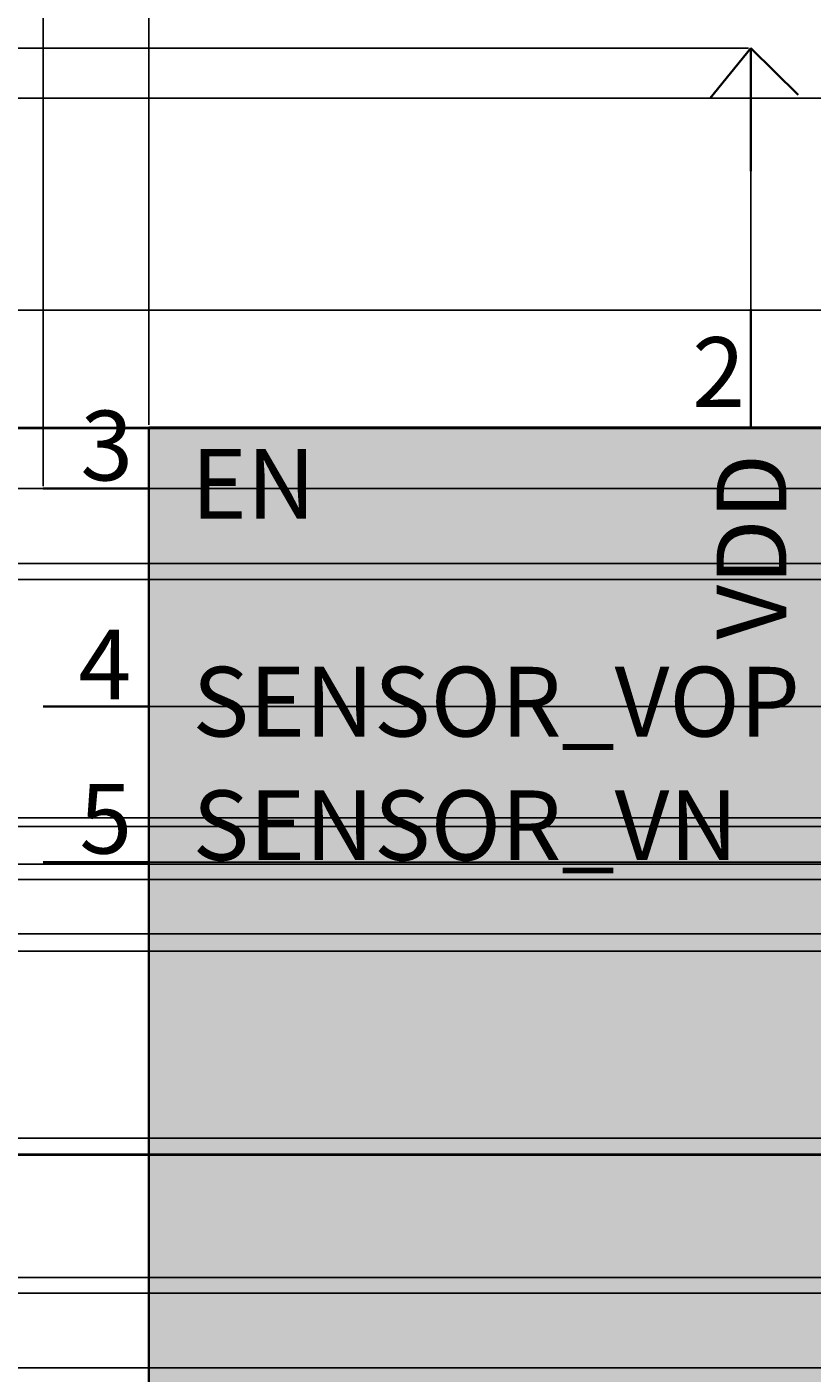
# Model space of a CAD drawing. Units: inches. Extents: x 23 to 132, y 5 to 105.
# Tile 4 of 14: x 47 to 66, y 54 to 87. Entities that reach past the tile are written whole.
import ezdxf

# ---------------------------------------------------------------- set-up
doc = ezdxf.new("R2010")
doc.units = ezdxf.units.IN
doc.header["$MEASUREMENT"] = 0
for name, color, linetype, lineweight in [('A-ANNO-DIMS', 2, 'Continuous', 18), ('E-ANNO-TEXT', 3, 'Continuous', 18), ('E-SYMB', 1, 'Continuous', 35), ('E-SYMB-PATT', 1, 'Continuous', 18), ('E-WIRE', 3, 'Continuous', 25)]:
    doc.layers.add(name, color=color, linetype=linetype, lineweight=lineweight)
doc.styles.get("Standard").update_dxf_attribs({"font": 'arial.ttf'})
doc.dimstyles.get("Standard").update_dxf_attribs({"dimtxt": 0.18, "dimasz": 0.18, "dimexe": 0.18, "dimexo": 0.0625, "dimgap": 0.09, "dimtad": 0, "dimtih": 1, "dimtoh": 1, "dimdec": 4, "dimzin": 0, "dimdsep": 46, "dimtxsty": 'Standard', "dimcen": 0.09, "dimadec": 0, "dimazin": 0, "dimtfac": 1, "dimtdec": 4, "dimtofl": 0, "dimtmove": 0, "dimatfit": 3, "dimfxl": 1, "dimtolj": 1, "dimtzin": 0, "dimarcsym": 0})

# ---------------------------------------------------------------- blocks, each defined once
blk = doc.blocks.new('*D2')
at = {"layer": 'A-ANNO-DIMS', "color": 0, "lineweight": -2, "transparency": 16777216}
for p, q in [((28.697, 66.272), (28.697, 105.232)), ((28.877, 105.052), (75.577, 105.052)), ((123.031, 105.052), (76.33, 105.052)), ((123.211, 99.539), (123.211, 105.232))]:
    blk.add_line(p, q, dxfattribs=at)
at = {"layer": 'A-ANNO-DIMS', "color": 0, "transparency": 16777216}
for points in [[(28.877, 105.082), (28.877, 105.022), (28.697, 105.052)], [(123.031, 105.082), (123.031, 105.022), (123.211, 105.052)]]:
    blk.add_solid(points, dxfattribs=at)
at = {"layer": 'Defpoints', "color": 0, "transparency": 16777216}
for p in [(123.211, 105.052), (123.211, 99.477), (28.697, 66.21)]:
    blk.add_point(p, dxfattribs=at)
at = {"layer": 'A-ANNO-DIMS', "color": 0, "transparency": 16777216, "insert": (75.954, 105.052), "char_height": 0.18, "attachment_point": 5}
blk.add_mtext('\\A1;94.51', dxfattribs=at)
blk = doc.blocks.new('*D6')
at = {"layer": 'A-ANNO-DIMS', "color": 0, "lineweight": -2, "transparency": 16777216}
for p, q in [((50.202, 77.095), (22.942, 77.095)), ((23.122, 76.915), (23.122, 47.733)), ((23.122, 18.187), (23.122, 47.369)), ((50.202, 18.007), (22.942, 18.007))]:
    blk.add_line(p, q, dxfattribs=at)
at = {"layer": 'A-ANNO-DIMS', "color": 0, "transparency": 16777216}
for points in [[(23.092, 76.915), (23.152, 76.915), (23.122, 77.095)], [(23.092, 18.187), (23.152, 18.187), (23.122, 18.007)]]:
    blk.add_solid(points, dxfattribs=at)
at = {"layer": 'Defpoints', "color": 0, "transparency": 16777216}
for p in [(23.122, 77.095), (50.265, 77.095), (50.265, 18.007)]:
    blk.add_point(p, dxfattribs=at)
at = {"layer": 'A-ANNO-DIMS', "color": 0, "transparency": 16777216, "insert": (23.122, 47.551), "char_height": 0.18, "attachment_point": 5}
blk.add_mtext('\\A1;59.09', dxfattribs=at)
blk = doc.blocks.new('*D7')
at = {"layer": 'A-ANNO-DIMS', "color": 0, "lineweight": -2, "transparency": 16777216}
for p, q in [((30.295, 73.877), (30.295, 105.232)), ((30.475, 105.052), (39.895, 105.052)), ((50.085, 105.052), (40.665, 105.052)), ((50.265, 77.157), (50.265, 105.232))]:
    blk.add_line(p, q, dxfattribs=at)
at = {"layer": 'A-ANNO-DIMS', "color": 0, "transparency": 16777216}
for points in [[(30.475, 105.082), (30.475, 105.022), (30.295, 105.052)], [(50.085, 105.082), (50.085, 105.022), (50.265, 105.052)]]:
    blk.add_solid(points, dxfattribs=at)
at = {"layer": 'Defpoints', "color": 0, "transparency": 16777216}
for p in [(50.265, 105.052), (50.265, 77.095), (30.295, 73.814)]:
    blk.add_point(p, dxfattribs=at)
at = {"layer": 'A-ANNO-DIMS', "color": 0, "transparency": 16777216, "insert": (40.28, 105.052), "char_height": 0.18, "attachment_point": 5}
blk.add_mtext('\\A1;19.97', dxfattribs=at)
blk = doc.blocks.new('*D12')
at = {"layer": 'A-ANNO-DIMS', "color": 0, "lineweight": -2, "transparency": 16777216}
for p, q in [((64.714, 86.23), (22.942, 86.23)), ((23.122, 86.05), (23.122, 81.845)), ((23.122, 77.275), (23.122, 81.481)), ((64.714, 77.095), (22.942, 77.095))]:
    blk.add_line(p, q, dxfattribs=at)
at = {"layer": 'A-ANNO-DIMS', "color": 0, "transparency": 16777216}
for points in [[(23.092, 86.05), (23.152, 86.05), (23.122, 86.23)], [(23.092, 77.275), (23.152, 77.275), (23.122, 77.095)]]:
    blk.add_solid(points, dxfattribs=at)
at = {"layer": 'Defpoints', "color": 0, "transparency": 16777216}
for p in [(23.122, 86.23), (64.777, 86.23), (64.777, 77.095)]:
    blk.add_point(p, dxfattribs=at)
at = {"layer": 'A-ANNO-DIMS', "color": 0, "transparency": 16777216, "insert": (23.122, 81.663), "char_height": 0.18, "attachment_point": 5}
blk.add_mtext('\\A1;9.135', dxfattribs=at)
blk = doc.blocks.new('*D15')
at = {"layer": 'A-ANNO-DIMS', "color": 0, "lineweight": -2, "transparency": 16777216}
for p, q in [((50.327, 77.095), (129.239, 77.095)), ((129.059, 76.915), (129.059, 76.538)), ((129.059, 75.801), (129.059, 76.177)), ((47.783, 75.621), (129.239, 75.621))]:
    blk.add_line(p, q, dxfattribs=at)
at = {"layer": 'A-ANNO-DIMS', "color": 0, "transparency": 16777216}
for points in [[(129.029, 76.915), (129.089, 76.915), (129.059, 77.095)], [(129.029, 75.801), (129.089, 75.801), (129.059, 75.621)]]:
    blk.add_solid(points, dxfattribs=at)
at = {"layer": 'Defpoints', "color": 0, "transparency": 16777216}
for p in [(50.265, 77.095), (47.72, 75.621), (129.059, 75.621)]:
    blk.add_point(p, dxfattribs=at)
at = {"layer": 'A-ANNO-DIMS', "color": 0, "transparency": 16777216, "insert": (129.059, 76.358), "char_height": 0.18, "attachment_point": 5}
blk.add_mtext('\\A1;1.47', dxfattribs=at)
blk = doc.blocks.new('*D16')
at = {"layer": 'A-ANNO-DIMS', "color": 0, "lineweight": -2, "transparency": 16777216}
for p, q in [((47.783, 75.621), (129.239, 75.621)), ((129.059, 75.441), (129.059, 73.177)), ((129.059, 70.55), (129.059, 72.814)), ((47.783, 70.37), (129.239, 70.37))]:
    blk.add_line(p, q, dxfattribs=at)
at = {"layer": 'A-ANNO-DIMS', "color": 0, "transparency": 16777216}
for points in [[(129.029, 75.441), (129.089, 75.441), (129.059, 75.621)], [(129.029, 70.55), (129.089, 70.55), (129.059, 70.37)]]:
    blk.add_solid(points, dxfattribs=at)
at = {"layer": 'Defpoints', "color": 0, "transparency": 16777216}
for p in [(47.72, 75.621), (47.72, 70.37), (129.059, 70.37)]:
    blk.add_point(p, dxfattribs=at)
at = {"layer": 'A-ANNO-DIMS', "color": 0, "transparency": 16777216, "insert": (129.059, 72.996), "char_height": 0.18, "attachment_point": 5}
blk.add_mtext('\\A1;5.25', dxfattribs=at)
blk = doc.blocks.new('*D17')
at = {"layer": 'A-ANNO-DIMS', "color": 0, "lineweight": -2, "transparency": 16777216}
for p, q in [((47.783, 70.37), (129.239, 70.37)), ((129.059, 70.19), (129.059, 68.678)), ((129.059, 66.801), (129.059, 68.314)), ((47.783, 66.621), (129.239, 66.621))]:
    blk.add_line(p, q, dxfattribs=at)
at = {"layer": 'A-ANNO-DIMS', "color": 0, "transparency": 16777216}
for points in [[(129.029, 70.19), (129.089, 70.19), (129.059, 70.37)], [(129.029, 66.801), (129.089, 66.801), (129.059, 66.621)]]:
    blk.add_solid(points, dxfattribs=at)
at = {"layer": 'Defpoints', "color": 0, "transparency": 16777216}
for p in [(47.72, 70.37), (47.72, 66.621), (129.059, 66.621)]:
    blk.add_point(p, dxfattribs=at)
at = {"layer": 'A-ANNO-DIMS', "color": 0, "transparency": 16777216, "insert": (129.059, 68.496), "char_height": 0.18, "attachment_point": 5}
blk.add_mtext('\\A1;3.75', dxfattribs=at)
blk = doc.blocks.new('*D48')
at = {"layer": 'A-ANNO-DIMS', "color": 0, "lineweight": -2, "transparency": 16777216}
for p, q in [((41.783, 75.637), (41.783, 105.232)), ((41.963, 105.052), (44.358, 105.052)), ((47.54, 105.052), (45.145, 105.052)), ((47.72, 75.683), (47.72, 105.232))]:
    blk.add_line(p, q, dxfattribs=at)
at = {"layer": 'A-ANNO-DIMS', "color": 0, "transparency": 16777216}
for points in [[(41.963, 105.082), (41.963, 105.022), (41.783, 105.052)], [(47.54, 105.082), (47.54, 105.022), (47.72, 105.052)]]:
    blk.add_solid(points, dxfattribs=at)
at = {"layer": 'Defpoints', "color": 0, "transparency": 16777216}
for p in [(47.72, 105.052), (41.783, 75.575), (47.72, 75.621)]:
    blk.add_point(p, dxfattribs=at)
at = {"layer": 'A-ANNO-DIMS', "color": 0, "transparency": 16777216, "insert": (44.752, 105.052), "char_height": 0.18, "attachment_point": 5}
blk.add_mtext('\\A1;5.937', dxfattribs=at)
blk = doc.blocks.new('*D57')
at = {"layer": 'A-ANNO-DIMS', "color": 0, "lineweight": -2, "transparency": 16777216}
for p, q in [((30.358, 64.901), (129.239, 64.901)), ((129.059, 64.721), (129.059, 62.62)), ((129.059, 60.155), (129.059, 62.256)), ((30.358, 59.975), (129.239, 59.975))]:
    blk.add_line(p, q, dxfattribs=at)
at = {"layer": 'A-ANNO-DIMS', "color": 0, "transparency": 16777216}
for points in [[(129.029, 64.721), (129.089, 64.721), (129.059, 64.901)], [(129.029, 60.155), (129.089, 60.155), (129.059, 59.975)]]:
    blk.add_solid(points, dxfattribs=at)
at = {"layer": 'Defpoints', "color": 0, "transparency": 16777216}
for p in [(30.295, 64.901), (129.059, 64.901), (30.295, 59.975)]:
    blk.add_point(p, dxfattribs=at)
at = {"layer": 'A-ANNO-DIMS', "color": 0, "transparency": 16777216, "insert": (129.059, 62.438), "char_height": 0.18, "attachment_point": 5}
blk.add_mtext('\\A1;4.925', dxfattribs=at)
blk = doc.blocks.new('*D58')
at = {"layer": 'A-ANNO-DIMS', "color": 0, "lineweight": -2, "transparency": 16777216}
for p, q in [((30.358, 73.814), (129.239, 73.814)), ((129.059, 73.634), (129.059, 70.194)), ((129.059, 66.39), (129.059, 69.83)), ((30.359, 66.21), (129.239, 66.21))]:
    blk.add_line(p, q, dxfattribs=at)
at = {"layer": 'A-ANNO-DIMS', "color": 0, "transparency": 16777216}
for points in [[(129.029, 73.634), (129.089, 73.634), (129.059, 73.814)], [(129.029, 66.39), (129.089, 66.39), (129.059, 66.21)]]:
    blk.add_solid(points, dxfattribs=at)
at = {"layer": 'Defpoints', "color": 0, "transparency": 16777216}
for p in [(30.295, 73.814), (129.059, 73.814), (30.297, 66.21)]:
    blk.add_point(p, dxfattribs=at)
at = {"layer": 'A-ANNO-DIMS', "color": 0, "transparency": 16777216, "insert": (129.059, 70.012), "char_height": 0.18, "attachment_point": 5}
blk.add_mtext('\\A1;7.604', dxfattribs=at)
blk = doc.blocks.new('*D65')
at = {"layer": 'A-ANNO-DIMS', "color": 0, "lineweight": -2, "transparency": 16777216}
for p, q in [((38.414, 67.485), (129.239, 67.485)), ((129.059, 67.305), (129.059, 66.165)), ((129.059, 64.66), (129.059, 65.801)), ((38.414, 64.48), (129.239, 64.48))]:
    blk.add_line(p, q, dxfattribs=at)
at = {"layer": 'A-ANNO-DIMS', "color": 0, "transparency": 16777216}
for points in [[(129.029, 67.305), (129.089, 67.305), (129.059, 67.485)], [(129.029, 64.66), (129.089, 64.66), (129.059, 64.48)]]:
    blk.add_solid(points, dxfattribs=at)
at = {"layer": 'Defpoints', "color": 0, "transparency": 16777216}
for p in [(38.351, 67.485), (129.059, 67.485), (38.351, 64.48)]:
    blk.add_point(p, dxfattribs=at)
at = {"layer": 'A-ANNO-DIMS', "color": 0, "transparency": 16777216, "insert": (129.059, 65.983), "char_height": 0.18, "attachment_point": 5}
blk.add_mtext('\\A1;3.005', dxfattribs=at)
blk = doc.blocks.new('*D70')
at = {"layer": 'A-ANNO-DIMS', "color": 0, "lineweight": -2, "transparency": 16777216}
for p, q in [((35.392, 56.625), (129.239, 56.625)), ((129.059, 56.445), (129.059, 55.716)), ((129.059, 54.624), (129.059, 55.352)), ((33.892, 54.444), (129.239, 54.444))]:
    blk.add_line(p, q, dxfattribs=at)
at = {"layer": 'A-ANNO-DIMS', "color": 0, "transparency": 16777216}
for points in [[(129.029, 56.445), (129.089, 56.445), (129.059, 56.625)], [(129.029, 54.624), (129.089, 54.624), (129.059, 54.444)]]:
    blk.add_solid(points, dxfattribs=at)
at = {"layer": 'Defpoints', "color": 0, "transparency": 16777216}
for p in [(35.33, 56.625), (33.83, 54.444), (129.059, 54.444)]:
    blk.add_point(p, dxfattribs=at)
at = {"layer": 'A-ANNO-DIMS', "color": 0, "transparency": 16777216, "insert": (129.059, 55.534), "char_height": 0.18, "attachment_point": 5}
blk.add_mtext('\\A1;2.18', dxfattribs=at)
blk = doc.blocks.new('*D78')
at = {"layer": 'A-ANNO-DIMS', "color": 0, "lineweight": -2, "transparency": 16777216}
for p, q in [((112.773, 67.688), (22.942, 67.688)), ((23.122, 67.508), (23.122, 67.314)), ((23.122, 66.759), (23.122, 66.953)), ((112.773, 66.579), (22.942, 66.579))]:
    blk.add_line(p, q, dxfattribs=at)
at = {"layer": 'A-ANNO-DIMS', "color": 0, "transparency": 16777216}
for points in [[(23.092, 67.508), (23.152, 67.508), (23.122, 67.688)], [(23.092, 66.759), (23.152, 66.759), (23.122, 66.579)]]:
    blk.add_solid(points, dxfattribs=at)
at = {"layer": 'Defpoints', "color": 0, "transparency": 16777216}
for p in [(23.122, 67.688), (112.835, 67.688), (112.835, 66.579)]:
    blk.add_point(p, dxfattribs=at)
at = {"layer": 'A-ANNO-DIMS', "color": 0, "transparency": 16777216, "insert": (23.122, 67.133), "char_height": 0.18, "attachment_point": 5}
blk.add_mtext('\\A1;1.11', dxfattribs=at)
blk = doc.blocks.new('*D79')
at = {"layer": 'A-ANNO-DIMS', "color": 0, "lineweight": -2, "transparency": 16777216}
for p, q in [((114.373, 66.579), (22.942, 66.579)), ((23.122, 66.399), (23.122, 63.267)), ((23.122, 59.77), (23.122, 62.903)), ((114.371, 59.59), (22.942, 59.59))]:
    blk.add_line(p, q, dxfattribs=at)
at = {"layer": 'A-ANNO-DIMS', "color": 0, "transparency": 16777216}
for points in [[(23.092, 66.399), (23.152, 66.399), (23.122, 66.579)], [(23.092, 59.77), (23.152, 59.77), (23.122, 59.59)]]:
    blk.add_solid(points, dxfattribs=at)
at = {"layer": 'Defpoints', "color": 0, "transparency": 16777216}
for p in [(23.122, 66.579), (114.435, 66.579), (114.434, 59.59)]:
    blk.add_point(p, dxfattribs=at)
at = {"layer": 'A-ANNO-DIMS', "color": 0, "transparency": 16777216, "insert": (23.122, 63.085), "char_height": 0.18, "attachment_point": 5}
blk.add_mtext('\\A1;6.988', dxfattribs=at)
blk = doc.blocks.new('*D80')
at = {"layer": 'A-ANNO-DIMS', "color": 0, "lineweight": -2, "transparency": 16777216}
for p, q in [((114.373, 73.429), (22.942, 73.429)), ((23.122, 73.249), (23.122, 70.741)), ((23.122, 67.868), (23.122, 70.377)), ((114.373, 67.688), (22.942, 67.688))]:
    blk.add_line(p, q, dxfattribs=at)
at = {"layer": 'A-ANNO-DIMS', "color": 0, "transparency": 16777216}
for points in [[(23.092, 73.249), (23.152, 73.249), (23.122, 73.429)], [(23.092, 67.868), (23.152, 67.868), (23.122, 67.688)]]:
    blk.add_solid(points, dxfattribs=at)
at = {"layer": 'Defpoints', "color": 0, "transparency": 16777216}
for p in [(23.122, 73.429), (114.435, 73.429), (114.435, 67.688)]:
    blk.add_point(p, dxfattribs=at)
at = {"layer": 'A-ANNO-DIMS', "color": 0, "transparency": 16777216, "insert": (23.122, 70.559), "char_height": 0.18, "attachment_point": 5}
blk.add_mtext('\\A1;5.741', dxfattribs=at)
blk = doc.blocks.new('*D81')
at = {"layer": 'A-ANNO-DIMS', "color": 0, "lineweight": -2, "transparency": 16777216}
for p, q in [((110.705, 59.566), (22.942, 59.566)), ((23.122, 59.386), (23.122, 58.085)), ((23.122, 56.42), (23.122, 57.721)), ((110.759, 56.24), (22.942, 56.24))]:
    blk.add_line(p, q, dxfattribs=at)
at = {"layer": 'A-ANNO-DIMS', "color": 0, "transparency": 16777216}
for points in [[(23.092, 59.386), (23.152, 59.386), (23.122, 59.566)], [(23.092, 56.42), (23.152, 56.42), (23.122, 56.24)]]:
    blk.add_solid(points, dxfattribs=at)
at = {"layer": 'Defpoints', "color": 0, "transparency": 16777216}
for p in [(23.122, 59.566), (110.768, 59.566), (110.822, 56.24)]:
    blk.add_point(p, dxfattribs=at)
at = {"layer": 'A-ANNO-DIMS', "color": 0, "transparency": 16777216, "insert": (23.122, 57.903), "char_height": 0.18, "attachment_point": 5}
blk.add_mtext('\\A1;3.326', dxfattribs=at)
blk = doc.blocks.new('*D85')
at = {"layer": 'A-ANNO-DIMS', "color": 0, "lineweight": -2, "transparency": 16777216}
for p, q in [((106.903, 97.776), (22.942, 97.776)), ((23.122, 97.596), (23.122, 87.606)), ((23.122, 77.251), (23.122, 87.242)), ((106.964, 77.071), (22.942, 77.071))]:
    blk.add_line(p, q, dxfattribs=at)
at = {"layer": 'A-ANNO-DIMS', "color": 0, "transparency": 16777216}
for points in [[(23.092, 97.596), (23.152, 97.596), (23.122, 97.776)], [(23.092, 77.251), (23.152, 77.251), (23.122, 77.071)]]:
    blk.add_solid(points, dxfattribs=at)
at = {"layer": 'Defpoints', "color": 0, "transparency": 16777216}
for p in [(23.122, 97.776), (106.965, 97.776), (107.026, 77.071)]:
    blk.add_point(p, dxfattribs=at)
at = {"layer": 'A-ANNO-DIMS', "color": 0, "transparency": 16777216, "insert": (23.122, 87.424), "char_height": 0.18, "attachment_point": 5}
blk.add_mtext('\\A1;20.705', dxfattribs=at)
blk = doc.blocks.new('*D86')
at = {"layer": 'A-ANNO-DIMS', "color": 0, "lineweight": -2, "transparency": 16777216}
for p, q in [((110.027, 79.916), (22.942, 79.916)), ((23.122, 79.736), (23.122, 78.675)), ((23.122, 77.251), (23.122, 78.312)), ((106.964, 77.071), (22.942, 77.071))]:
    blk.add_line(p, q, dxfattribs=at)
at = {"layer": 'A-ANNO-DIMS', "color": 0, "transparency": 16777216}
for points in [[(23.092, 79.736), (23.152, 79.736), (23.122, 79.916)], [(23.092, 77.251), (23.152, 77.251), (23.122, 77.071)]]:
    blk.add_solid(points, dxfattribs=at)
at = {"layer": 'Defpoints', "color": 0, "transparency": 16777216}
for p in [(23.122, 79.916), (110.089, 79.916), (107.026, 77.071)]:
    blk.add_point(p, dxfattribs=at)
at = {"layer": 'A-ANNO-DIMS', "color": 0, "transparency": 16777216, "insert": (23.122, 78.493), "char_height": 0.18, "attachment_point": 5}
blk.add_mtext('\\A1;2.84', dxfattribs=at)
blk = doc.blocks.new('*D87')
at = {"layer": 'A-ANNO-DIMS', "color": 0, "lineweight": -2, "transparency": 16777216}
for p, q in [((110.027, 85.021), (22.942, 85.021)), ((23.122, 84.841), (23.122, 82.65)), ((23.122, 80.096), (23.122, 82.286)), ((110.027, 79.916), (22.942, 79.916))]:
    blk.add_line(p, q, dxfattribs=at)
at = {"layer": 'A-ANNO-DIMS', "color": 0, "transparency": 16777216}
for points in [[(23.092, 84.841), (23.152, 84.841), (23.122, 85.021)], [(23.092, 80.096), (23.152, 80.096), (23.122, 79.916)]]:
    blk.add_solid(points, dxfattribs=at)
at = {"layer": 'Defpoints', "color": 0, "transparency": 16777216}
for p in [(23.122, 85.021), (110.089, 85.021), (110.089, 79.916)]:
    blk.add_point(p, dxfattribs=at)
at = {"layer": 'A-ANNO-DIMS', "color": 0, "transparency": 16777216, "insert": (23.122, 82.468), "char_height": 0.18, "attachment_point": 5}
blk.add_mtext('\\A1;5.105', dxfattribs=at)
blk = doc.blocks.new('*D88')
at = {"layer": 'A-ANNO-DIMS', "color": 0, "lineweight": -2, "transparency": 16777216}
for p, q in [((110.027, 89.722), (22.942, 89.722)), ((23.122, 89.542), (23.122, 87.554)), ((23.122, 85.201), (23.122, 87.19)), ((110.027, 85.021), (22.942, 85.021))]:
    blk.add_line(p, q, dxfattribs=at)
at = {"layer": 'A-ANNO-DIMS', "color": 0, "transparency": 16777216}
for points in [[(23.092, 89.542), (23.152, 89.542), (23.122, 89.722)], [(23.092, 85.201), (23.152, 85.201), (23.122, 85.021)]]:
    blk.add_solid(points, dxfattribs=at)
at = {"layer": 'Defpoints', "color": 0, "transparency": 16777216}
for p in [(23.122, 89.722), (110.089, 89.722), (110.089, 85.021)]:
    blk.add_point(p, dxfattribs=at)
at = {"layer": 'A-ANNO-DIMS', "color": 0, "transparency": 16777216, "insert": (23.122, 87.372), "char_height": 0.18, "attachment_point": 5}
blk.add_mtext('\\A1;4.702', dxfattribs=at)

msp = doc.modelspace()

# ---------------------------------------------------------------- hatches: boundary and pattern name
at = {"layer": 'E-SYMB-PATT'}
h = msp.add_hatch(color=256, dxfattribs=at)
h.dxf.hatch_style = 1
h.paths.add_polyline_path([(80.9692, 77.095), (50.2646, 77.095), (50.2646, 18.0066), (80.9692, 18.0066)])

# ---------------------------------------------------------------- linework, layer by layer
at = {"layer": 'E-SYMB'}
for p, q in [((64.7769, 86.2302), (63.7949, 85.0212)), ((64.7769, 83.2684), (64.7769, 86.2302)), ((64.7769, 86.2302), (65.9155, 85.1012)), ((64.7769, 77.095), (64.7769, 79.9458)), ((47.7202, 75.6207), (50.2646, 75.6207)), ((47.7202, 70.3705), (50.2646, 70.3705)), ((47.7202, 66.621), (50.2646, 66.621))]:
    msp.add_line(p, q, dxfattribs=at)
msp.add_lwpolyline([(50.2646, 77.095), (80.9692, 77.095), (80.9692, 18.0066), (50.2646, 18.0066)], close=True, dxfattribs=at)
at = {"layer": 'E-WIRE'}
for p, q in [((64.7769, 79.9458), (64.7769, 83.2684)), ((47.7202, 75.6207), (37.4432, 75.6207))]:
    msp.add_line(p, q, dxfattribs=at)

# ---------------------------------------------------------------- texts
at = {"layer": 'E-ANNO-TEXT'}
for s, height, p in [('2', 1.6794, (63.3621, 77.587)), ('3', 1.6794, (48.6142, 75.8177)), ('EN', 1.67943, (51.2785, 74.8944)), ('4', 1.6794, (48.5676, 70.5438)), ('SENSOR_VOP', 1.67943, (51.3182, 69.6493)), ('5', 1.6794, (48.5907, 66.8308)), ('SENSOR_VN', 1.67943, (51.3182, 66.6726))]:
    msp.add_text(s, height=height, dxfattribs=at).set_placement(p)
msp.add_text('VDD', height=1.67943, rotation=90, dxfattribs=at).set_placement((65.6289, 71.9842))

# ---------------------------------------------------------------- dimensions: what is measured, and where the dimension line sits
at = {"layer": 'A-ANNO-DIMS'}
for base, p1, p2, override, picture, middle in [((123.2107, 105.052), (28.6965, 66.2099), (123.2107, 99.477), {"dimdec": 2, "dimlfac": 1, "dimrnd": 0, "dimzin": 0, "dimdsep": 46, "dimlunit": 2}, '*D2', (75.9536, 105.052)), ((50.2646, 105.052), (30.2954, 73.8144), (50.2646, 77.095), {"dimdec": 2, "dimlfac": 1, "dimrnd": 0, "dimzin": 0, "dimdsep": 46, "dimlunit": 2}, '*D7', (40.28, 105.052)), ((47.7202, 105.052), (41.7829, 75.5745), (47.7202, 75.6207), {"dimdec": 3, "dimlfac": 1, "dimrnd": 0, "dimzin": 0, "dimdsep": 46, "dimlunit": 2}, '*D48', (44.7515, 105.052))]:
    dim = msp.add_linear_dim(base=base, p1=p1, p2=p2, dimstyle='Standard', override=override, dxfattribs=at)
    dim.commit()
    dim.dimension.update_dxf_attribs({"geometry": picture, "text_midpoint": middle})
for base, p1, p2, override, picture, middle in [((23.1215, 97.7764), (107.026, 77.0711), (106.9652, 97.7764), {"dimdec": 3, "dimlfac": 1, "dimrnd": 0, "dimzin": 0, "dimdsep": 46, "dimlunit": 2}, '*D85', (23.1215, 87.4238)), ((23.12152, 89.7224), (110.08916, 85.02085), (110.08916, 89.7224), {"dimdec": 3, "dimlfac": 1, "dimrnd": 0, "dimzin": 0, "dimdsep": 46, "dimlunit": 2}, '*D88', (23.12152, 87.37162)), ((23.1215, 86.2302), (64.7769, 77.095), (64.7769, 86.2302), {"dimdec": 3, "dimlfac": 1, "dimrnd": 0, "dimzin": 0, "dimdsep": 46, "dimlunit": 2}, '*D12', (23.1215, 81.6626)), ((23.1215, 85.0209), (110.0892, 79.9158), (110.0892, 85.0209), {"dimdec": 3, "dimlfac": 1, "dimrnd": 0, "dimzin": 0, "dimdsep": 46, "dimlunit": 2}, '*D87', (23.1215, 82.4683)), ((23.1215, 79.9158), (107.026, 77.0711), (110.0892, 79.9158), {"dimdec": 2, "dimlfac": 1, "dimrnd": 0, "dimzin": 0, "dimdsep": 46, "dimlunit": 2}, '*D86', (23.1215, 78.4935)), ((23.1215, 77.095), (50.2646, 18.0066), (50.2646, 77.095), {"dimdec": 2, "dimlfac": 1, "dimrnd": 0, "dimzin": 0, "dimdsep": 46, "dimlunit": 2}, '*D6', (23.1215, 47.5508)), ((129.0589, 75.6207), (50.2646, 77.095), (47.7202, 75.6207), {"dimdec": 2, "dimlfac": 1, "dimrnd": 0, "dimzin": 0, "dimdsep": 46, "dimlunit": 2}, '*D15', (129.0589, 76.3579)), ((129.0589, 70.3705), (47.7202, 75.6207), (47.7202, 70.3705), {"dimdec": 2, "dimlfac": 1, "dimrnd": 0, "dimzin": 0, "dimdsep": 46, "dimlunit": 2}, '*D16', (129.0589, 72.9956)), ((129.05891, 73.81438), (30.29652, 66.20989), (30.29537, 73.81438), {"dimdec": 3, "dimlfac": 1, "dimrnd": 0, "dimzin": 0, "dimdsep": 46, "dimlunit": 2}, '*D58', (129.05891, 70.01213)), ((23.1215, 73.4293), (114.4351, 67.6881), (114.4351, 73.4293), {"dimdec": 3, "dimlfac": 1, "dimrnd": 0, "dimzin": 0, "dimdsep": 46, "dimlunit": 2}, '*D80', (23.1215, 70.5587)), ((129.0589, 66.621), (47.7202, 70.3705), (47.7202, 66.621), {"dimdec": 2, "dimlfac": 1, "dimrnd": 0, "dimzin": 0, "dimdsep": 46, "dimlunit": 2}, '*D17', (129.0589, 68.4957)), ((23.1215, 67.6881), (112.8351, 66.5788), (112.8351, 67.6881), {"dimdec": 2, "dimlfac": 1, "dimrnd": 0, "dimzin": 0, "dimdsep": 46, "dimlunit": 2}, '*D78', (23.1215, 67.1334)), ((129.0589, 67.4851), (38.3512, 64.4801), (38.3512, 67.4851), {"dimdec": 3, "dimlfac": 1, "dimrnd": 0, "dimzin": 0, "dimdsep": 46, "dimlunit": 2}, '*D65', (129.0589, 65.9826)), ((23.1215, 66.5788), (114.434, 59.5904), (114.4351, 66.5788), {"dimdec": 3, "dimlfac": 1, "dimrnd": 0, "dimzin": 0, "dimdsep": 46, "dimlunit": 2}, '*D79', (23.1215, 63.0846)), ((129.0589, 64.9007), (30.2954, 59.9755), (30.2954, 64.9007), {"dimdec": 3, "dimlfac": 1, "dimrnd": 0, "dimzin": 0, "dimdsep": 46, "dimlunit": 2}, '*D57', (129.0589, 62.4381)), ((23.1215, 59.566), (110.8219, 56.2399), (110.7677, 59.566), {"dimdec": 3, "dimlfac": 1, "dimrnd": 0, "dimzin": 0, "dimdsep": 46, "dimlunit": 2}, '*D81', (23.1215, 57.9029)), ((129.0589, 54.4437), (35.3299, 56.6249), (33.8299, 54.4437), {"dimdec": 2, "dimlfac": 1, "dimrnd": 0, "dimzin": 0, "dimdsep": 46, "dimlunit": 2}, '*D70', (129.0589, 55.5343))]:
    dim = msp.add_linear_dim(base=base, p1=p1, p2=p2, angle=90, dimstyle='Standard', override=override, dxfattribs=at)
    dim.commit()
    dim.dimension.update_dxf_attribs({"geometry": picture, "text_midpoint": middle})

doc.saveas('drawing.dxf')
